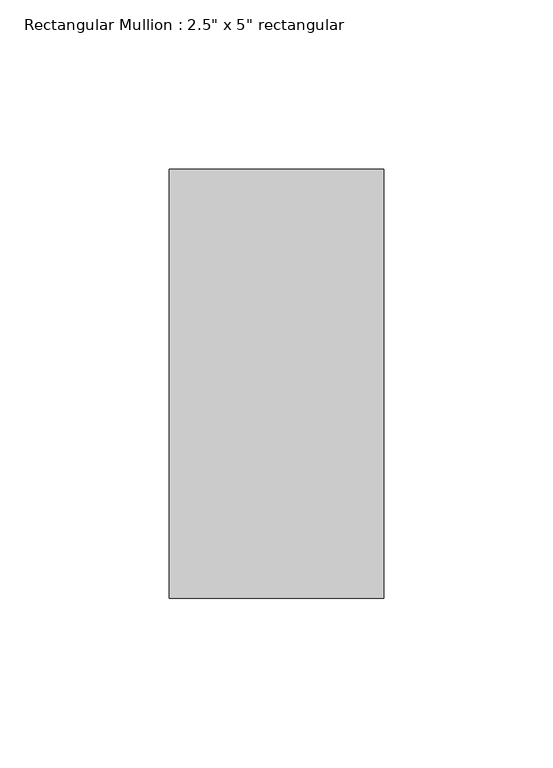
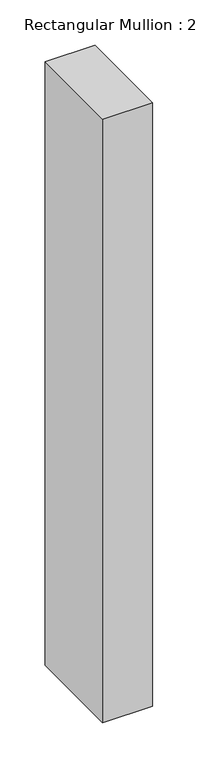
"""IFC4 building model written with IfcOpenShell, lengths in millimetres: member geometry."""

from ifc_helpers import new_model, si_unit, frame, origin, place, context, project, spatial, polyline, outline, extrude, source, transform, mapped, element, save


def member_58a4a87b(model_context):
    return source(origin(), model_context, "Body", "SweptSolid", [
        extrude(outline(polyline([(31.75, 63.5), (31.75, -63.5), (-31.75, -63.5), (-31.75, 63.5), (31.75, 63.5)])), frame((0.0, 0.0, -812.8), z_axis=(0.0, 0.0, 1.0), x_axis=(1.0, 0.0, 0.0)), (0.0, 0.0, 1.0), 812.8),
    ])


if __name__ == "__main__":
    model = new_model("IFC4")
    model_context = context("Model", 3, world=origin())
    ifc_project = project(units=[si_unit("LENGTHUNIT", "METRE", prefix="MILLI")], contexts=[model_context])
    site = spatial("IfcSite", under=ifc_project)
    building = spatial("IfcBuilding", under=site)
    placement = place(None, origin())
    member_shape = member_58a4a87b(model_context)
    element("IfcMember", 1, ObjectType="Rectangular Mullion : 2.5\" x 5\" rectangular", at=placement, inside=building, context=model_context, shape_type="MappedRepresentation", body=[
        mapped(member_shape, transform((0.0, 0.0, 0.0), x_axis=(1.0, 0.0, 0.0), y_axis=(0.0, 1.0, 0.0), z_axis=(0.0, 0.0, 1.0))),
    ])
    save(model, "model.ifc")

# Revit data of these elements
# Type "Rectangular Mullion : 2.5\" x 5\" rectangular"
#   built-in parameter 1007304 = 0.416667 (stored number, unit not read)
#   built-in parameter 1007301 = 0.104167 (stored number, unit not read)
#   built-in parameter 1007300 = 0.104167 (stored number, unit not read)
